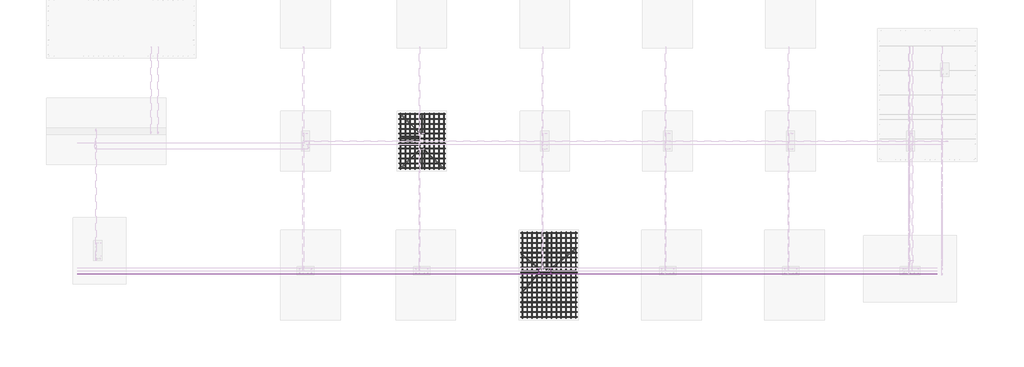
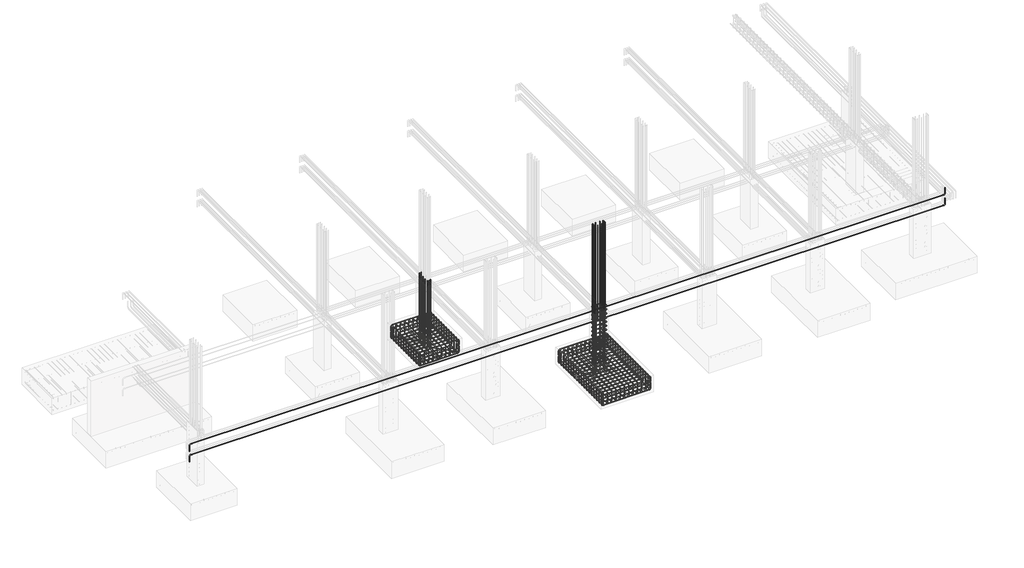
# One storey, part 5 of 18: 30 reinforcing bars.
"""IFC4 building model written with IfcOpenShell, lengths in millimetres."""

from ifc_helpers import new_model, si_unit, point, frame, origin, place, context, project, spatial, polyline, circle_curve, trimmed, segment, composite_curve, source, transform, mapped, element, save
from ifc_brep_helpers import swept_disk

model = new_model("IFC4")

# Units and contexts
model_context = context("Model", 3, world=origin())
ifc_project = project(units=[si_unit("LENGTHUNIT", "METRE", prefix="MILLI")], contexts=[model_context])

# Site, building, storey
site = spatial("IfcSite", under=ifc_project)
building = spatial("IfcBuilding", under=site)
storey = spatial("IfcBuildingStorey", under=building, Elevation=-2000.0)

# Reinforcing bars
placement = place(None, origin())
reinforcing_bar_shape = source(origin(), model_context, "Body", "SolidModel", [
    swept_disk(composite_curve([segment(polyline([(-4478.5399692, -834.8555128, -2300.0), (-4478.5399692, -834.8555128, -2486.6)]), True, "CONTINUOUS"), segment(trimmed(circle_curve(frame((-4533.9899692, -834.8555128, -2486.6), z_axis=(0.0, 1.0, 0.0), x_axis=(55.44999999999982, 0.0, 0.0)), 55.45), [point((-4478.5399692, -834.8555128, -2486.6))], [point((-4533.9899692, -834.8555128, -2542.05))], True, "CARTESIAN"), True, "CONTINUOUS"), segment(polyline([(-4533.9899692, -834.8555128, -2542.05), (-5807.1899692, -834.8555128, -2542.05)]), True, "CONTINUOUS"), segment(trimmed(circle_curve(frame((-5807.1899692, -834.8555128, -2486.6), z_axis=(0.0, 1.0, 0.0), x_axis=(0.0, 0.0, -55.45000000000027)), 55.45), [point((-5807.1899692, -834.8555128, -2542.05))], [point((-5862.6399692, -834.8555128, -2486.6))], True, "CARTESIAN"), True, "CONTINUOUS"), segment(polyline([(-5862.6399692, -834.8555128, -2486.6), (-5862.6399692, -834.8555128, -2300.0)]), True, "CONTINUOUS")], self_intersect=False), 7.95),
])
element("IfcReinforcingBar", 1, at=placement, inside=storey, context=model_context, shape_type="MappedRepresentation", body=[
    mapped(reinforcing_bar_shape, transform((0.0, 0.0, 0.0), x_axis=(1.0, 0.0, 0.0), y_axis=(0.0, 1.0, 0.0), z_axis=(0.0, 0.0, 1.0))),
    mapped(reinforcing_bar_shape, transform((0.0, -148.4250709, 0.0), x_axis=(1.0, 0.0, 0.0), y_axis=(0.0, 1.0, 0.0), z_axis=(0.0, 0.0, 1.0))),
    mapped(reinforcing_bar_shape, transform((0.0, -296.8501418, 0.0), x_axis=(1.0, 0.0, 0.0), y_axis=(0.0, 1.0, 0.0), z_axis=(0.0, 0.0, 1.0))),
    mapped(reinforcing_bar_shape, transform((0.0, -445.2752126, 0.0), x_axis=(1.0, 0.0, 0.0), y_axis=(0.0, 1.0, 0.0), z_axis=(0.0, 0.0, 1.0))),
    mapped(reinforcing_bar_shape, transform((0.0, -593.7002835, 0.0), x_axis=(1.0, 0.0, 0.0), y_axis=(0.0, 1.0, 0.0), z_axis=(0.0, 0.0, 1.0))),
    mapped(reinforcing_bar_shape, transform((0.0, -742.1253544, 0.0), x_axis=(1.0, 0.0, 0.0), y_axis=(0.0, 1.0, 0.0), z_axis=(0.0, 0.0, 1.0))),
    mapped(reinforcing_bar_shape, transform((0.0, -890.5504253, 0.0), x_axis=(1.0, 0.0, 0.0), y_axis=(0.0, 1.0, 0.0), z_axis=(0.0, 0.0, 1.0))),
    mapped(reinforcing_bar_shape, transform((0.0, -1038.9754961, 0.0), x_axis=(1.0, 0.0, 0.0), y_axis=(0.0, 1.0, 0.0), z_axis=(0.0, 0.0, 1.0))),
    mapped(reinforcing_bar_shape, transform((0.0, -1187.400567, 0.0), x_axis=(1.0, 0.0, 0.0), y_axis=(0.0, 1.0, 0.0), z_axis=(0.0, 0.0, 1.0))),
    mapped(reinforcing_bar_shape, transform((0.0, -1335.8256379, 0.0), x_axis=(1.0, 0.0, 0.0), y_axis=(0.0, 1.0, 0.0), z_axis=(0.0, 0.0, 1.0))),
    mapped(reinforcing_bar_shape, transform((0.0, -1484.2507088, 0.0), x_axis=(1.0, 0.0, 0.0), y_axis=(0.0, 1.0, 0.0), z_axis=(0.0, 0.0, 1.0))),
    mapped(reinforcing_bar_shape, transform((0.0, -1632.6757796, 0.0), x_axis=(1.0, 0.0, 0.0), y_axis=(0.0, 1.0, 0.0), z_axis=(0.0, 0.0, 1.0))),
])
reinforcing_bar_2_shape = source(origin(), model_context, "Body", "SolidModel", [
    swept_disk(composite_curve([segment(polyline([(-5864.5899692, -834.8555128, -2250.0), (-5864.5899692, -834.8555128, -2102.0)]), True, "CONTINUOUS"), segment(trimmed(circle_curve(frame((-5818.5899692, -834.8555128, -2102.0), z_axis=(0.0, 1.0, 0.0), x_axis=(-46.0, 0.0, 0.0)), 46.0), [point((-5864.5899692, -834.8555128, -2102.0))], [point((-5818.5899692, -834.8555128, -2056.0))], True, "CARTESIAN"), True, "CONTINUOUS"), segment(polyline([(-5818.5899692, -834.8555128, -2056.0), (-4522.5899692, -834.8555128, -2056.0)]), True, "CONTINUOUS"), segment(trimmed(circle_curve(frame((-4522.5899692, -834.8555128, -2102.0), z_axis=(0.0, 1.0, 0.0), x_axis=(0.0, 0.0, 46.0)), 46.0), [point((-4522.5899692, -834.8555128, -2056.0))], [point((-4476.5899692, -834.8555128, -2102.0))], True, "CARTESIAN"), True, "CONTINUOUS"), segment(polyline([(-4476.5899692, -834.8555128, -2102.0), (-4476.5899692, -834.8555128, -2250.0)]), True, "CONTINUOUS")], self_intersect=False), 6.0),
])
element("IfcReinforcingBar", 2, at=placement, inside=storey, context=model_context, shape_type="MappedRepresentation", body=[
    mapped(reinforcing_bar_2_shape, transform((0.0, 0.0, 0.0), x_axis=(1.0, 0.0, 0.0), y_axis=(0.0, 1.0, 0.0), z_axis=(0.0, 0.0, 1.0))),
    mapped(reinforcing_bar_2_shape, transform((0.0, -148.4250709, 0.0), x_axis=(1.0, 0.0, 0.0), y_axis=(0.0, 1.0, 0.0), z_axis=(0.0, 0.0, 1.0))),
    mapped(reinforcing_bar_2_shape, transform((0.0, -296.8501418, 0.0), x_axis=(1.0, 0.0, 0.0), y_axis=(0.0, 1.0, 0.0), z_axis=(0.0, 0.0, 1.0))),
    mapped(reinforcing_bar_2_shape, transform((0.0, -445.2752126, 0.0), x_axis=(1.0, 0.0, 0.0), y_axis=(0.0, 1.0, 0.0), z_axis=(0.0, 0.0, 1.0))),
    mapped(reinforcing_bar_2_shape, transform((0.0, -593.7002835, 0.0), x_axis=(1.0, 0.0, 0.0), y_axis=(0.0, 1.0, 0.0), z_axis=(0.0, 0.0, 1.0))),
    mapped(reinforcing_bar_2_shape, transform((0.0, -742.1253544, 0.0), x_axis=(1.0, 0.0, 0.0), y_axis=(0.0, 1.0, 0.0), z_axis=(0.0, 0.0, 1.0))),
    mapped(reinforcing_bar_2_shape, transform((0.0, -890.5504253, 0.0), x_axis=(1.0, 0.0, 0.0), y_axis=(0.0, 1.0, 0.0), z_axis=(0.0, 0.0, 1.0))),
    mapped(reinforcing_bar_2_shape, transform((0.0, -1038.9754961, 0.0), x_axis=(1.0, 0.0, 0.0), y_axis=(0.0, 1.0, 0.0), z_axis=(0.0, 0.0, 1.0))),
    mapped(reinforcing_bar_2_shape, transform((0.0, -1187.400567, 0.0), x_axis=(1.0, 0.0, 0.0), y_axis=(0.0, 1.0, 0.0), z_axis=(0.0, 0.0, 1.0))),
    mapped(reinforcing_bar_2_shape, transform((0.0, -1335.8256379, 0.0), x_axis=(1.0, 0.0, 0.0), y_axis=(0.0, 1.0, 0.0), z_axis=(0.0, 0.0, 1.0))),
    mapped(reinforcing_bar_2_shape, transform((0.0, -1484.2507088, 0.0), x_axis=(1.0, 0.0, 0.0), y_axis=(0.0, 1.0, 0.0), z_axis=(0.0, 0.0, 1.0))),
    mapped(reinforcing_bar_2_shape, transform((0.0, -1632.6757796, 0.0), x_axis=(1.0, 0.0, 0.0), y_axis=(0.0, 1.0, 0.0), z_axis=(0.0, 0.0, 1.0))),
])
reinforcing_bar_3_shape = source(origin(), model_context, "Body", "SolidModel", [
    swept_disk(composite_curve([segment(polyline([(-5818.4091864, -811.9600376, -2322.6684255), (-5818.4091864, -811.9600376, -2470.6684255)]), True, "CONTINUOUS"), segment(trimmed(circle_curve(frame((-5818.4091864, -857.9600376, -2470.6684255), z_axis=(-1.0, 0.0, 0.0), x_axis=(0.0, 46.0, 0.0)), 46.0), [point((-5818.4091864, -811.9600376, -2470.6684255))], [point((-5818.4091864, -857.9600376, -2516.6684255))], True, "CARTESIAN"), True, "CONTINUOUS"), segment(polyline([(-5818.4091864, -857.9600376, -2516.6684255), (-5818.4091864, -2453.9600376, -2516.6684255)]), True, "CONTINUOUS"), segment(trimmed(circle_curve(frame((-5818.4091864, -2453.9600376, -2470.6684255), z_axis=(-1.0, 0.0, 0.0), x_axis=(0.0, 0.0, -46.0)), 46.0), [point((-5818.4091864, -2453.9600376, -2516.6684255))], [point((-5818.4091864, -2499.9600376, -2470.6684255))], True, "CARTESIAN"), True, "CONTINUOUS"), segment(polyline([(-5818.4091864, -2499.9600376, -2470.6684255), (-5818.4091864, -2499.9600376, -2322.6684255)]), True, "CONTINUOUS")], self_intersect=False), 6.0),
])
element("IfcReinforcingBar", 3, at=placement, inside=storey, context=model_context, shape_type="MappedRepresentation", body=[
    mapped(reinforcing_bar_3_shape, transform((0.0, 0.0, 0.0), x_axis=(1.0, 0.0, 0.0), y_axis=(0.0, 1.0, 0.0), z_axis=(0.0, 0.0, 1.0))),
    mapped(reinforcing_bar_3_shape, transform((144.8687847, 0.0, 0.0), x_axis=(1.0, 0.0, 0.0), y_axis=(0.0, 1.0, 0.0), z_axis=(0.0, 0.0, 1.0))),
    mapped(reinforcing_bar_3_shape, transform((289.7375694, 0.0, 0.0), x_axis=(1.0, 0.0, 0.0), y_axis=(0.0, 1.0, 0.0), z_axis=(0.0, 0.0, 1.0))),
    mapped(reinforcing_bar_3_shape, transform((434.6063541, 0.0, 0.0), x_axis=(1.0, 0.0, 0.0), y_axis=(0.0, 1.0, 0.0), z_axis=(0.0, 0.0, 1.0))),
    mapped(reinforcing_bar_3_shape, transform((579.4751388, 0.0, 0.0), x_axis=(1.0, 0.0, 0.0), y_axis=(0.0, 1.0, 0.0), z_axis=(0.0, 0.0, 1.0))),
    mapped(reinforcing_bar_3_shape, transform((724.3439235, 0.0, 0.0), x_axis=(1.0, 0.0, 0.0), y_axis=(0.0, 1.0, 0.0), z_axis=(0.0, 0.0, 1.0))),
    mapped(reinforcing_bar_3_shape, transform((869.2127082, 0.0, 0.0), x_axis=(1.0, 0.0, 0.0), y_axis=(0.0, 1.0, 0.0), z_axis=(0.0, 0.0, 1.0))),
    mapped(reinforcing_bar_3_shape, transform((1014.0814929, 0.0, 0.0), x_axis=(1.0, 0.0, 0.0), y_axis=(0.0, 1.0, 0.0), z_axis=(0.0, 0.0, 1.0))),
    mapped(reinforcing_bar_3_shape, transform((1158.9502776, 0.0, 0.0), x_axis=(1.0, 0.0, 0.0), y_axis=(0.0, 1.0, 0.0), z_axis=(0.0, 0.0, 1.0))),
    mapped(reinforcing_bar_3_shape, transform((1303.8190623, 0.0, 0.0), x_axis=(1.0, 0.0, 0.0), y_axis=(0.0, 1.0, 0.0), z_axis=(0.0, 0.0, 1.0))),
])
reinforcing_bar_4_shape = source(origin(), model_context, "Body", "SolidModel", [
    swept_disk(composite_curve([segment(polyline([(-4512.6669522, -811.9600376, -2276.6677805), (-4512.6669522, -811.9600376, -2128.6677805)]), True, "CONTINUOUS"), segment(trimmed(circle_curve(frame((-4512.6669522, -857.9600376, -2128.6677805), z_axis=(1.0, 0.0, 0.0), x_axis=(0.0, 46.0, 0.0)), 46.0), [point((-4512.6669522, -811.9600376, -2128.6677805))], [point((-4512.6669522, -857.9600376, -2082.6677805))], True, "CARTESIAN"), True, "CONTINUOUS"), segment(polyline([(-4512.6669522, -857.9600376, -2082.6677805), (-4512.6669522, -2453.9600376, -2082.6677805)]), True, "CONTINUOUS"), segment(trimmed(circle_curve(frame((-4512.6669522, -2453.9600376, -2128.6677805), z_axis=(1.0, 0.0, 0.0), x_axis=(0.0, 0.0, 46.0)), 46.0), [point((-4512.6669522, -2453.9600376, -2082.6677805))], [point((-4512.6669522, -2499.9600376, -2128.6677805))], True, "CARTESIAN"), True, "CONTINUOUS"), segment(polyline([(-4512.6669522, -2499.9600376, -2128.6677805), (-4512.6669522, -2499.9600376, -2276.6677805)]), True, "CONTINUOUS")], self_intersect=False), 6.0),
])
element("IfcReinforcingBar", 4, at=placement, inside=storey, context=model_context, shape_type="MappedRepresentation", body=[
    mapped(reinforcing_bar_4_shape, transform((0.0, 0.0, 0.0), x_axis=(1.0, 0.0, 0.0), y_axis=(0.0, 1.0, 0.0), z_axis=(0.0, 0.0, 1.0))),
    mapped(reinforcing_bar_4_shape, transform((-145.0824705, 0.0, 0.0), x_axis=(1.0, 0.0, 0.0), y_axis=(0.0, 1.0, 0.0), z_axis=(0.0, 0.0, 1.0))),
    mapped(reinforcing_bar_4_shape, transform((-290.1649409, 0.0, 0.0), x_axis=(1.0, 0.0, 0.0), y_axis=(0.0, 1.0, 0.0), z_axis=(0.0, 0.0, 1.0))),
    mapped(reinforcing_bar_4_shape, transform((-435.2474114, 0.0, 0.0), x_axis=(1.0, 0.0, 0.0), y_axis=(0.0, 1.0, 0.0), z_axis=(0.0, 0.0, 1.0))),
    mapped(reinforcing_bar_4_shape, transform((-580.3298819, 0.0, 0.0), x_axis=(1.0, 0.0, 0.0), y_axis=(0.0, 1.0, 0.0), z_axis=(0.0, 0.0, 1.0))),
    mapped(reinforcing_bar_4_shape, transform((-725.4123523, 0.0, 0.0), x_axis=(1.0, 0.0, 0.0), y_axis=(0.0, 1.0, 0.0), z_axis=(0.0, 0.0, 1.0))),
    mapped(reinforcing_bar_4_shape, transform((-870.4948228, 0.0, 0.0), x_axis=(1.0, 0.0, 0.0), y_axis=(0.0, 1.0, 0.0), z_axis=(0.0, 0.0, 1.0))),
    mapped(reinforcing_bar_4_shape, transform((-1015.5772932, 0.0, 0.0), x_axis=(1.0, 0.0, 0.0), y_axis=(0.0, 1.0, 0.0), z_axis=(0.0, 0.0, 1.0))),
    mapped(reinforcing_bar_4_shape, transform((-1160.6597637, 0.0, 0.0), x_axis=(1.0, 0.0, 0.0), y_axis=(0.0, 1.0, 0.0), z_axis=(0.0, 0.0, 1.0))),
    mapped(reinforcing_bar_4_shape, transform((-1305.7422342, 0.0, 0.0), x_axis=(1.0, 0.0, 0.0), y_axis=(0.0, 1.0, 0.0), z_axis=(0.0, 0.0, 1.0))),
])
reinforcing_bar_5_shape = source(origin(), model_context, "Body", "SolidModel", [
    swept_disk(composite_curve([segment(polyline([(-508.2940057, -4415.5752408, -2300.0), (-508.2940057, -4415.5752408, -2486.6)]), True, "CONTINUOUS"), segment(trimmed(circle_curve(frame((-563.7440057, -4415.5752408, -2486.6), z_axis=(0.0, 1.0, 0.0), x_axis=(55.44999999999999, 0.0, 0.0)), 55.45), [point((-508.2940057, -4415.5752408, -2486.6))], [point((-563.7440057, -4415.5752408, -2542.05))], True, "CARTESIAN"), True, "CONTINUOUS"), segment(polyline([(-563.7440057, -4415.5752408, -2542.05), (-2136.9440057, -4415.5752408, -2542.05)]), True, "CONTINUOUS"), segment(trimmed(circle_curve(frame((-2136.9440057, -4415.5752408, -2486.6), z_axis=(0.0, 1.0, 0.0), x_axis=(0.0, 0.0, -55.45000000000027)), 55.45), [point((-2136.9440057, -4415.5752408, -2542.05))], [point((-2192.3940057, -4415.5752408, -2486.6))], True, "CARTESIAN"), True, "CONTINUOUS"), segment(polyline([(-2192.3940057, -4415.5752408, -2486.6), (-2192.3940057, -4415.5752408, -2300.0)]), True, "CONTINUOUS")], self_intersect=False), 7.95),
])
element("IfcReinforcingBar", 5, at=placement, inside=storey, context=model_context, shape_type="MappedRepresentation", body=[
    mapped(reinforcing_bar_5_shape, transform((0.0, 0.0, 0.0), x_axis=(1.0, 0.0, 0.0), y_axis=(0.0, 1.0, 0.0), z_axis=(0.0, 0.0, 1.0))),
    mapped(reinforcing_bar_5_shape, transform((0.0, -148.9809282, 0.0), x_axis=(1.0, 0.0, 0.0), y_axis=(0.0, 1.0, 0.0), z_axis=(0.0, 0.0, 1.0))),
    mapped(reinforcing_bar_5_shape, transform((0.0, -297.9618564, 0.0), x_axis=(1.0, 0.0, 0.0), y_axis=(0.0, 1.0, 0.0), z_axis=(0.0, 0.0, 1.0))),
    mapped(reinforcing_bar_5_shape, transform((0.0, -446.9427846, 0.0), x_axis=(1.0, 0.0, 0.0), y_axis=(0.0, 1.0, 0.0), z_axis=(0.0, 0.0, 1.0))),
    mapped(reinforcing_bar_5_shape, transform((0.0, -595.9237129, 0.0), x_axis=(1.0, 0.0, 0.0), y_axis=(0.0, 1.0, 0.0), z_axis=(0.0, 0.0, 1.0))),
    mapped(reinforcing_bar_5_shape, transform((0.0, -744.9046411, 0.0), x_axis=(1.0, 0.0, 0.0), y_axis=(0.0, 1.0, 0.0), z_axis=(0.0, 0.0, 1.0))),
    mapped(reinforcing_bar_5_shape, transform((0.0, -893.8855693, 0.0), x_axis=(1.0, 0.0, 0.0), y_axis=(0.0, 1.0, 0.0), z_axis=(0.0, 0.0, 1.0))),
    mapped(reinforcing_bar_5_shape, transform((0.0, -1042.8664975, 0.0), x_axis=(1.0, 0.0, 0.0), y_axis=(0.0, 1.0, 0.0), z_axis=(0.0, 0.0, 1.0))),
    mapped(reinforcing_bar_5_shape, transform((0.0, -1191.8474257, 0.0), x_axis=(1.0, 0.0, 0.0), y_axis=(0.0, 1.0, 0.0), z_axis=(0.0, 0.0, 1.0))),
    mapped(reinforcing_bar_5_shape, transform((0.0, -1340.8283539, 0.0), x_axis=(1.0, 0.0, 0.0), y_axis=(0.0, 1.0, 0.0), z_axis=(0.0, 0.0, 1.0))),
    mapped(reinforcing_bar_5_shape, transform((0.0, -1489.8092821, 0.0), x_axis=(1.0, 0.0, 0.0), y_axis=(0.0, 1.0, 0.0), z_axis=(0.0, 0.0, 1.0))),
    mapped(reinforcing_bar_5_shape, transform((0.0, -1638.7902103, 0.0), x_axis=(1.0, 0.0, 0.0), y_axis=(0.0, 1.0, 0.0), z_axis=(0.0, 0.0, 1.0))),
    mapped(reinforcing_bar_5_shape, transform((0.0, -1787.7711386, 0.0), x_axis=(1.0, 0.0, 0.0), y_axis=(0.0, 1.0, 0.0), z_axis=(0.0, 0.0, 1.0))),
    mapped(reinforcing_bar_5_shape, transform((0.0, -1936.7520668, 0.0), x_axis=(1.0, 0.0, 0.0), y_axis=(0.0, 1.0, 0.0), z_axis=(0.0, 0.0, 1.0))),
    mapped(reinforcing_bar_5_shape, transform((0.0, -2085.732995, 0.0), x_axis=(1.0, 0.0, 0.0), y_axis=(0.0, 1.0, 0.0), z_axis=(0.0, 0.0, 1.0))),
    mapped(reinforcing_bar_5_shape, transform((0.0, -2234.7139232, 0.0), x_axis=(1.0, 0.0, 0.0), y_axis=(0.0, 1.0, 0.0), z_axis=(0.0, 0.0, 1.0))),
    mapped(reinforcing_bar_5_shape, transform((0.0, -2383.6948514, 0.0), x_axis=(1.0, 0.0, 0.0), y_axis=(0.0, 1.0, 0.0), z_axis=(0.0, 0.0, 1.0))),
    mapped(reinforcing_bar_5_shape, transform((0.0, -2532.6757796, 0.0), x_axis=(1.0, 0.0, 0.0), y_axis=(0.0, 1.0, 0.0), z_axis=(0.0, 0.0, 1.0))),
])
reinforcing_bar_6_shape = source(origin(), model_context, "Body", "SolidModel", [
    swept_disk(composite_curve([segment(polyline([(-2194.3440057, -4415.5752408, -2250.0), (-2194.3440057, -4415.5752408, -2102.0)]), True, "CONTINUOUS"), segment(trimmed(circle_curve(frame((-2148.3440057, -4415.5752408, -2102.0), z_axis=(0.0, 1.0, 0.0), x_axis=(-46.0, 0.0, 0.0)), 46.0), [point((-2194.3440057, -4415.5752408, -2102.0))], [point((-2148.3440057, -4415.5752408, -2056.0))], True, "CARTESIAN"), True, "CONTINUOUS"), segment(polyline([(-2148.3440057, -4415.5752408, -2056.0), (-552.3440057, -4415.5752408, -2056.0)]), True, "CONTINUOUS"), segment(trimmed(circle_curve(frame((-552.3440057, -4415.5752408, -2102.0), z_axis=(0.0, 1.0, 0.0), x_axis=(0.0, 0.0, 46.0)), 46.0), [point((-552.3440057, -4415.5752408, -2056.0))], [point((-506.3440057, -4415.5752408, -2102.0))], True, "CARTESIAN"), True, "CONTINUOUS"), segment(polyline([(-506.3440057, -4415.5752408, -2102.0), (-506.3440057, -4415.5752408, -2250.0)]), True, "CONTINUOUS")], self_intersect=False), 6.0),
])
element("IfcReinforcingBar", 6, at=placement, inside=storey, context=model_context, shape_type="MappedRepresentation", body=[
    mapped(reinforcing_bar_6_shape, transform((0.0, 0.0, 0.0), x_axis=(1.0, 0.0, 0.0), y_axis=(0.0, 1.0, 0.0), z_axis=(0.0, 0.0, 1.0))),
    mapped(reinforcing_bar_6_shape, transform((0.0, -148.9809282, 0.0), x_axis=(1.0, 0.0, 0.0), y_axis=(0.0, 1.0, 0.0), z_axis=(0.0, 0.0, 1.0))),
    mapped(reinforcing_bar_6_shape, transform((0.0, -297.9618564, 0.0), x_axis=(1.0, 0.0, 0.0), y_axis=(0.0, 1.0, 0.0), z_axis=(0.0, 0.0, 1.0))),
    mapped(reinforcing_bar_6_shape, transform((0.0, -446.9427846, 0.0), x_axis=(1.0, 0.0, 0.0), y_axis=(0.0, 1.0, 0.0), z_axis=(0.0, 0.0, 1.0))),
    mapped(reinforcing_bar_6_shape, transform((0.0, -595.9237129, 0.0), x_axis=(1.0, 0.0, 0.0), y_axis=(0.0, 1.0, 0.0), z_axis=(0.0, 0.0, 1.0))),
    mapped(reinforcing_bar_6_shape, transform((0.0, -744.9046411, 0.0), x_axis=(1.0, 0.0, 0.0), y_axis=(0.0, 1.0, 0.0), z_axis=(0.0, 0.0, 1.0))),
    mapped(reinforcing_bar_6_shape, transform((0.0, -893.8855693, 0.0), x_axis=(1.0, 0.0, 0.0), y_axis=(0.0, 1.0, 0.0), z_axis=(0.0, 0.0, 1.0))),
    mapped(reinforcing_bar_6_shape, transform((0.0, -1042.8664975, 0.0), x_axis=(1.0, 0.0, 0.0), y_axis=(0.0, 1.0, 0.0), z_axis=(0.0, 0.0, 1.0))),
    mapped(reinforcing_bar_6_shape, transform((0.0, -1191.8474257, 0.0), x_axis=(1.0, 0.0, 0.0), y_axis=(0.0, 1.0, 0.0), z_axis=(0.0, 0.0, 1.0))),
    mapped(reinforcing_bar_6_shape, transform((0.0, -1340.8283539, 0.0), x_axis=(1.0, 0.0, 0.0), y_axis=(0.0, 1.0, 0.0), z_axis=(0.0, 0.0, 1.0))),
    mapped(reinforcing_bar_6_shape, transform((0.0, -1489.8092821, 0.0), x_axis=(1.0, 0.0, 0.0), y_axis=(0.0, 1.0, 0.0), z_axis=(0.0, 0.0, 1.0))),
    mapped(reinforcing_bar_6_shape, transform((0.0, -1638.7902103, 0.0), x_axis=(1.0, 0.0, 0.0), y_axis=(0.0, 1.0, 0.0), z_axis=(0.0, 0.0, 1.0))),
    mapped(reinforcing_bar_6_shape, transform((0.0, -1787.7711386, 0.0), x_axis=(1.0, 0.0, 0.0), y_axis=(0.0, 1.0, 0.0), z_axis=(0.0, 0.0, 1.0))),
    mapped(reinforcing_bar_6_shape, transform((0.0, -1936.7520668, 0.0), x_axis=(1.0, 0.0, 0.0), y_axis=(0.0, 1.0, 0.0), z_axis=(0.0, 0.0, 1.0))),
    mapped(reinforcing_bar_6_shape, transform((0.0, -2085.732995, 0.0), x_axis=(1.0, 0.0, 0.0), y_axis=(0.0, 1.0, 0.0), z_axis=(0.0, 0.0, 1.0))),
    mapped(reinforcing_bar_6_shape, transform((0.0, -2234.7139232, 0.0), x_axis=(1.0, 0.0, 0.0), y_axis=(0.0, 1.0, 0.0), z_axis=(0.0, 0.0, 1.0))),
    mapped(reinforcing_bar_6_shape, transform((0.0, -2383.6948514, 0.0), x_axis=(1.0, 0.0, 0.0), y_axis=(0.0, 1.0, 0.0), z_axis=(0.0, 0.0, 1.0))),
    mapped(reinforcing_bar_6_shape, transform((0.0, -2532.6757796, 0.0), x_axis=(1.0, 0.0, 0.0), y_axis=(0.0, 1.0, 0.0), z_axis=(0.0, 0.0, 1.0))),
])
reinforcing_bar_7_shape = source(origin(), model_context, "Body", "SolidModel", [
    swept_disk(composite_curve([segment(polyline([(-2148.1632229, -4392.6797656, -2322.6684255), (-2148.1632229, -4392.6797656, -2470.6684255)]), True, "CONTINUOUS"), segment(trimmed(circle_curve(frame((-2148.1632229, -4438.6797656, -2470.6684255), z_axis=(-1.0, 0.0, 0.0), x_axis=(0.0, 46.0, 0.0)), 46.0), [point((-2148.1632229, -4392.6797656, -2470.6684255))], [point((-2148.1632229, -4438.6797656, -2516.6684255))], True, "CARTESIAN"), True, "CONTINUOUS"), segment(polyline([(-2148.1632229, -4438.6797656, -2516.6684255), (-2148.1632229, -6934.6797656, -2516.6684255)]), True, "CONTINUOUS"), segment(trimmed(circle_curve(frame((-2148.1632229, -6934.6797656, -2470.6684255), z_axis=(-1.0, 0.0, 0.0), x_axis=(0.0, 0.0, -46.0)), 46.0), [point((-2148.1632229, -6934.6797656, -2516.6684255))], [point((-2148.1632229, -6980.6797656, -2470.6684255))], True, "CARTESIAN"), True, "CONTINUOUS"), segment(polyline([(-2148.1632229, -6980.6797656, -2470.6684255), (-2148.1632229, -6980.6797656, -2322.6684255)]), True, "CONTINUOUS")], self_intersect=False), 6.0),
])
element("IfcReinforcingBar", 7, at=placement, inside=storey, context=model_context, shape_type="MappedRepresentation", body=[
    mapped(reinforcing_bar_7_shape, transform((0.0, 0.0, 0.0), x_axis=(1.0, 0.0, 0.0), y_axis=(0.0, 1.0, 0.0), z_axis=(0.0, 0.0, 1.0))),
    mapped(reinforcing_bar_7_shape, transform((145.8017329, 0.0, 0.0), x_axis=(1.0, 0.0, 0.0), y_axis=(0.0, 1.0, 0.0), z_axis=(0.0, 0.0, 1.0))),
    mapped(reinforcing_bar_7_shape, transform((291.6034659, 0.0, 0.0), x_axis=(1.0, 0.0, 0.0), y_axis=(0.0, 1.0, 0.0), z_axis=(0.0, 0.0, 1.0))),
    mapped(reinforcing_bar_7_shape, transform((437.4051988, 0.0, 0.0), x_axis=(1.0, 0.0, 0.0), y_axis=(0.0, 1.0, 0.0), z_axis=(0.0, 0.0, 1.0))),
    mapped(reinforcing_bar_7_shape, transform((583.2069318, 0.0, 0.0), x_axis=(1.0, 0.0, 0.0), y_axis=(0.0, 1.0, 0.0), z_axis=(0.0, 0.0, 1.0))),
    mapped(reinforcing_bar_7_shape, transform((729.0086647, 0.0, 0.0), x_axis=(1.0, 0.0, 0.0), y_axis=(0.0, 1.0, 0.0), z_axis=(0.0, 0.0, 1.0))),
    mapped(reinforcing_bar_7_shape, transform((874.8103976, 0.0, 0.0), x_axis=(1.0, 0.0, 0.0), y_axis=(0.0, 1.0, 0.0), z_axis=(0.0, 0.0, 1.0))),
    mapped(reinforcing_bar_7_shape, transform((1020.6121306, 0.0, 0.0), x_axis=(1.0, 0.0, 0.0), y_axis=(0.0, 1.0, 0.0), z_axis=(0.0, 0.0, 1.0))),
    mapped(reinforcing_bar_7_shape, transform((1166.4138635, 0.0, 0.0), x_axis=(1.0, 0.0, 0.0), y_axis=(0.0, 1.0, 0.0), z_axis=(0.0, 0.0, 1.0))),
    mapped(reinforcing_bar_7_shape, transform((1312.2155965, 0.0, 0.0), x_axis=(1.0, 0.0, 0.0), y_axis=(0.0, 1.0, 0.0), z_axis=(0.0, 0.0, 1.0))),
    mapped(reinforcing_bar_7_shape, transform((1458.0173294, 0.0, 0.0), x_axis=(1.0, 0.0, 0.0), y_axis=(0.0, 1.0, 0.0), z_axis=(0.0, 0.0, 1.0))),
    mapped(reinforcing_bar_7_shape, transform((1603.8190623, 0.0, 0.0), x_axis=(1.0, 0.0, 0.0), y_axis=(0.0, 1.0, 0.0), z_axis=(0.0, 0.0, 1.0))),
])
reinforcing_bar_8_shape = source(origin(), model_context, "Body", "SolidModel", [
    swept_disk(composite_curve([segment(polyline([(-542.4209887, -4392.6797656, -2276.6677805), (-542.4209887, -4392.6797656, -2128.6677805)]), True, "CONTINUOUS"), segment(trimmed(circle_curve(frame((-542.4209887, -4438.6797656, -2128.6677805), z_axis=(1.0, 0.0, 0.0), x_axis=(0.0, 46.0, 0.0)), 46.0), [point((-542.4209887, -4392.6797656, -2128.6677805))], [point((-542.4209887, -4438.6797656, -2082.6677805))], True, "CARTESIAN"), True, "CONTINUOUS"), segment(polyline([(-542.4209887, -4438.6797656, -2082.6677805), (-542.4209887, -6934.6797656, -2082.6677805)]), True, "CONTINUOUS"), segment(trimmed(circle_curve(frame((-542.4209887, -6934.6797656, -2128.6677805), z_axis=(1.0, 0.0, 0.0), x_axis=(0.0, 0.0, 46.0)), 46.0), [point((-542.4209887, -6934.6797656, -2082.6677805))], [point((-542.4209887, -6980.6797656, -2128.6677805))], True, "CARTESIAN"), True, "CONTINUOUS"), segment(polyline([(-542.4209887, -6980.6797656, -2128.6677805), (-542.4209887, -6980.6797656, -2276.6677805)]), True, "CONTINUOUS")], self_intersect=False), 6.0),
])
element("IfcReinforcingBar", 8, at=placement, inside=storey, context=model_context, shape_type="MappedRepresentation", body=[
    mapped(reinforcing_bar_8_shape, transform((0.0, 0.0, 0.0), x_axis=(1.0, 0.0, 0.0), y_axis=(0.0, 1.0, 0.0), z_axis=(0.0, 0.0, 1.0))),
    mapped(reinforcing_bar_8_shape, transform((-145.9765667, 0.0, 0.0), x_axis=(1.0, 0.0, 0.0), y_axis=(0.0, 1.0, 0.0), z_axis=(0.0, 0.0, 1.0))),
    mapped(reinforcing_bar_8_shape, transform((-291.9531335, 0.0, 0.0), x_axis=(1.0, 0.0, 0.0), y_axis=(0.0, 1.0, 0.0), z_axis=(0.0, 0.0, 1.0))),
    mapped(reinforcing_bar_8_shape, transform((-437.9297002, 0.0, 0.0), x_axis=(1.0, 0.0, 0.0), y_axis=(0.0, 1.0, 0.0), z_axis=(0.0, 0.0, 1.0))),
    mapped(reinforcing_bar_8_shape, transform((-583.906267, 0.0, 0.0), x_axis=(1.0, 0.0, 0.0), y_axis=(0.0, 1.0, 0.0), z_axis=(0.0, 0.0, 1.0))),
    mapped(reinforcing_bar_8_shape, transform((-729.8828337, 0.0, 0.0), x_axis=(1.0, 0.0, 0.0), y_axis=(0.0, 1.0, 0.0), z_axis=(0.0, 0.0, 1.0))),
    mapped(reinforcing_bar_8_shape, transform((-875.8594005, 0.0, 0.0), x_axis=(1.0, 0.0, 0.0), y_axis=(0.0, 1.0, 0.0), z_axis=(0.0, 0.0, 1.0))),
    mapped(reinforcing_bar_8_shape, transform((-1021.8359672, 0.0, 0.0), x_axis=(1.0, 0.0, 0.0), y_axis=(0.0, 1.0, 0.0), z_axis=(0.0, 0.0, 1.0))),
    mapped(reinforcing_bar_8_shape, transform((-1167.8125339, 0.0, 0.0), x_axis=(1.0, 0.0, 0.0), y_axis=(0.0, 1.0, 0.0), z_axis=(0.0, 0.0, 1.0))),
    mapped(reinforcing_bar_8_shape, transform((-1313.7891007, 0.0, 0.0), x_axis=(1.0, 0.0, 0.0), y_axis=(0.0, 1.0, 0.0), z_axis=(0.0, 0.0, 1.0))),
    mapped(reinforcing_bar_8_shape, transform((-1459.7656674, 0.0, 0.0), x_axis=(1.0, 0.0, 0.0), y_axis=(0.0, 1.0, 0.0), z_axis=(0.0, 0.0, 1.0))),
    mapped(reinforcing_bar_8_shape, transform((-1605.7422342, 0.0, 0.0), x_axis=(1.0, 0.0, 0.0), y_axis=(0.0, 1.0, 0.0), z_axis=(0.0, 0.0, 1.0))),
])
reinforcing_bar_9_shape = source(origin(), model_context, "Body", "SolidModel", [
    swept_disk(composite_curve([segment(polyline([(-1360.4315175, -5535.5091206, -34.0), (-1304.0960659, -5479.1736689, -34.0)]), True, "CONTINUOUS"), segment(trimmed(circle_curve(frame((-1283.5899692, -5499.6797656, -34.0), z_axis=(0.0, 0.0, -1.0), x_axis=(-20.506096699999944, 20.506096699999944, 0.0)), 29.0), [point((-1304.0960659, -5479.1736689, -34.0))], [point((-1254.5899692, -5499.6797656, -34.0))], True, "CARTESIAN"), True, "CONTINUOUS"), segment(polyline([(-1254.5899692, -5499.6797656, -34.0), (-1254.5899692, -5623.6797656, -34.0)]), True, "CONTINUOUS"), segment(trimmed(circle_curve(frame((-1283.5899692, -5623.6797656, -34.0), z_axis=(0.0, 0.0, -1.0), x_axis=(29.0, 0.0, 0.0)), 29.0), [point((-1254.5899692, -5623.6797656, -34.0))], [point((-1283.5899692, -5652.6797656, -34.0))], True, "CARTESIAN"), True, "CONTINUOUS"), segment(polyline([(-1283.5899692, -5652.6797656, -34.0), (-1657.5899692, -5652.6797656, -34.0)]), True, "CONTINUOUS"), segment(trimmed(circle_curve(frame((-1657.5899692, -5623.707741, -32.7265044), z_axis=(0.0, 0.043913640913297095, -0.9990353307775146), x_axis=(0.0, -28.972024599999713, -1.2734955999999968)), 29.0), [point((-1657.5899692, -5652.6797656, -34.0))], [point((-1686.5899692, -5623.707741, -32.7265044))], True, "CARTESIAN"), True, "CONTINUOUS"), segment(polyline([(-1686.5899692, -5623.707741, -32.7265044), (-1686.5899692, -5499.6517902, -27.2734956)]), True, "CONTINUOUS"), segment(trimmed(circle_curve(frame((-1657.5899692, -5499.6517902, -27.2734956), z_axis=(0.0, 0.043913640913297095, -0.9990353307775146), x_axis=(-29.0, 0.0, 0.0)), 29.0), [point((-1686.5899692, -5499.6517902, -27.2734956))], [point((-1657.5899692, -5470.6797656, -26.0))], True, "CARTESIAN"), True, "CONTINUOUS"), segment(polyline([(-1657.5899692, -5470.6797656, -26.0), (-1283.5899692, -5470.6797656, -26.0)]), True, "CONTINUOUS"), segment(trimmed(circle_curve(frame((-1283.5899692, -5499.6797656, -26.0), z_axis=(0.0, 0.0, -1.0), x_axis=(0.0, 29.0, 0.0)), 29.0), [point((-1283.5899692, -5470.6797656, -26.0))], [point((-1263.0838726, -5520.1858622, -26.0))], True, "CARTESIAN"), True, "CONTINUOUS"), segment(polyline([(-1263.0838726, -5520.1858622, -26.0), (-1319.4193242, -5576.5213139, -26.0)]), True, "CONTINUOUS")], self_intersect=False), 4.0),
])
element("IfcReinforcingBar", 9, at=placement, inside=storey, context=model_context, shape_type="MappedRepresentation", body=[
    mapped(reinforcing_bar_9_shape, transform((0.0, 0.0, 0.0), x_axis=(1.0, 0.0, 0.0), y_axis=(0.0, 1.0, 0.0), z_axis=(0.0, 0.0, 1.0))),
    mapped(reinforcing_bar_9_shape, transform((0.0, 0.0, -148.6153846), x_axis=(1.0, 0.0, 0.0), y_axis=(0.0, 1.0, 0.0), z_axis=(0.0, 0.0, 1.0))),
    mapped(reinforcing_bar_9_shape, transform((0.0, 0.0, -297.2307692), x_axis=(1.0, 0.0, 0.0), y_axis=(0.0, 1.0, 0.0), z_axis=(0.0, 0.0, 1.0))),
    mapped(reinforcing_bar_9_shape, transform((0.0, 0.0, -445.8461538), x_axis=(1.0, 0.0, 0.0), y_axis=(0.0, 1.0, 0.0), z_axis=(0.0, 0.0, 1.0))),
    mapped(reinforcing_bar_9_shape, transform((0.0, 0.0, -594.4615385), x_axis=(1.0, 0.0, 0.0), y_axis=(0.0, 1.0, 0.0), z_axis=(0.0, 0.0, 1.0))),
    mapped(reinforcing_bar_9_shape, transform((0.0, 0.0, -743.0769231), x_axis=(1.0, 0.0, 0.0), y_axis=(0.0, 1.0, 0.0), z_axis=(0.0, 0.0, 1.0))),
    mapped(reinforcing_bar_9_shape, transform((0.0, 0.0, -891.6923077), x_axis=(1.0, 0.0, 0.0), y_axis=(0.0, 1.0, 0.0), z_axis=(0.0, 0.0, 1.0))),
    mapped(reinforcing_bar_9_shape, transform((0.0, 0.0, -1040.3076923), x_axis=(1.0, 0.0, 0.0), y_axis=(0.0, 1.0, 0.0), z_axis=(0.0, 0.0, 1.0))),
    mapped(reinforcing_bar_9_shape, transform((0.0, 0.0, -1188.9230769), x_axis=(1.0, 0.0, 0.0), y_axis=(0.0, 1.0, 0.0), z_axis=(0.0, 0.0, 1.0))),
    mapped(reinforcing_bar_9_shape, transform((0.0, 0.0, -1337.5384615), x_axis=(1.0, 0.0, 0.0), y_axis=(0.0, 1.0, 0.0), z_axis=(0.0, 0.0, 1.0))),
    mapped(reinforcing_bar_9_shape, transform((0.0, 0.0, -1486.1538462), x_axis=(1.0, 0.0, 0.0), y_axis=(0.0, 1.0, 0.0), z_axis=(0.0, 0.0, 1.0))),
    mapped(reinforcing_bar_9_shape, transform((0.0, 0.0, -1634.7692308), x_axis=(1.0, 0.0, 0.0), y_axis=(0.0, 1.0, 0.0), z_axis=(0.0, 0.0, 1.0))),
    mapped(reinforcing_bar_9_shape, transform((0.0, 0.0, -1783.3846154), x_axis=(1.0, 0.0, 0.0), y_axis=(0.0, 1.0, 0.0), z_axis=(0.0, 0.0, 1.0))),
    mapped(reinforcing_bar_9_shape, transform((0.0, 0.0, -1932.0), x_axis=(1.0, 0.0, 0.0), y_axis=(0.0, 1.0, 0.0), z_axis=(0.0, 0.0, 1.0))),
])
element("IfcReinforcingBar", 10, at=placement, inside=storey, context=model_context, shape_type="SolidModel", body=[
    swept_disk(composite_curve([segment(polyline([(-2173.6233429, -5063.6864072, -2480.0), (-1700.4558049, -5460.7211138, -2480.0)]), True, "CONTINUOUS"), segment(trimmed(circle_curve(frame((-1700.4558049, -5460.7211138, -2412.5), z_axis=(-0.6427876096865429, -0.766044443118975, 0.0), x_axis=(0.0, 0.0, -67.5)), 67.5), [point((-1700.4558049, -5460.7211138, -2480.0))], [point((-1648.747805, -5504.1092774, -2412.5))], True, "CARTESIAN"), True, "CONTINUOUS"), segment(polyline([(-1648.747805, -5504.1092774, -2412.5), (-1648.747805, -5504.1092774, -20.0)]), True, "CONTINUOUS")], self_intersect=False), 10.0),
])
element("IfcReinforcingBar", 11, at=placement, inside=storey, context=model_context, shape_type="SolidModel", body=[
    swept_disk(composite_curve([segment(polyline([(-2177.6576621, -5559.3632831, -2480.0), (-1705.107931, -5559.3632831, -2480.0)]), True, "CONTINUOUS"), segment(trimmed(circle_curve(frame((-1705.107931, -5559.3632831, -2434.0), z_axis=(0.0, -1.0, 0.0), x_axis=(0.0, 0.0, -46.0)), 46.0), [point((-1705.107931, -5559.3632831, -2480.0))], [point((-1659.107931, -5559.3632831, -2434.0))], True, "CARTESIAN"), True, "CONTINUOUS"), segment(polyline([(-1659.107931, -5559.3632831, -2434.0), (-1659.107931, -5559.3632831, -30.0)]), True, "CONTINUOUS")], self_intersect=False), 6.0),
])
element("IfcReinforcingBar", 12, at=placement, inside=storey, context=model_context, shape_type="SolidModel", body=[
    swept_disk(composite_curve([segment(polyline([(-527.0646685, -4861.8897199, -2480.0), (-1240.7241336, -5460.7211138, -2480.0)]), True, "CONTINUOUS"), segment(trimmed(circle_curve(frame((-1240.7241336, -5460.7211138, -2412.5), z_axis=(-0.6427876096865429, 0.766044443118975, 0.0), x_axis=(0.0, 0.0, -67.5)), 67.5), [point((-1240.7241336, -5460.7211138, -2480.0))], [point((-1292.4321335, -5504.1092774, -2412.5))], True, "CARTESIAN"), True, "CONTINUOUS"), segment(polyline([(-1292.4321335, -5504.1092774, -2412.5), (-1292.4321335, -5504.1092774, -20.0)]), True, "CONTINUOUS")], self_intersect=False), 10.0),
])
element("IfcReinforcingBar", 13, at=placement, inside=storey, context=model_context, shape_type="SolidModel", body=[
    swept_disk(composite_curve([segment(polyline([(-2180.6241894, -6231.1040429, -2480.0), (-1693.0317894, -5670.1931504, -2480.0)]), True, "CONTINUOUS"), segment(trimmed(circle_curve(frame((-1693.0317894, -5670.1931504, -2412.5), z_axis=(0.7547095802227678, -0.6560590289905122, 0.0), x_axis=(0.0, 0.0, -67.5)), 67.5), [point((-1693.0317894, -5670.1931504, -2480.0))], [point((-1648.747805, -5619.2502537, -2412.5))], True, "CARTESIAN"), True, "CONTINUOUS"), segment(polyline([(-1648.747805, -5619.2502537, -2412.5), (-1648.747805, -5619.2502537, -20.0)]), True, "CONTINUOUS")], self_intersect=False), 10.0),
])
element("IfcReinforcingBar", 14, at=placement, inside=storey, context=model_context, shape_type="SolidModel", body=[
    swept_disk(composite_curve([segment(polyline([(-523.0303493, -5559.3632831, -2480.0), (-1236.0720074, -5559.3632831, -2480.0)]), True, "CONTINUOUS"), segment(trimmed(circle_curve(frame((-1236.0720074, -5559.3632831, -2434.0), z_axis=(0.0, 1.0, 0.0), x_axis=(0.0, 0.0, -46.0)), 46.0), [point((-1236.0720074, -5559.3632831, -2480.0))], [point((-1282.0720074, -5559.3632831, -2434.0))], True, "CARTESIAN"), True, "CONTINUOUS"), segment(polyline([(-1282.0720074, -5559.3632831, -2434.0), (-1282.0720074, -5559.3632831, -30.0)]), True, "CONTINUOUS")], self_intersect=False), 6.0),
])
reinforcing_bar_10_shape = source(origin(), model_context, "Body", "SolidModel", [
    swept_disk(composite_curve([segment(polyline([(-1543.6420643, -4416.634351, -2480.0), (-1543.6420643, -5449.6419331, -2480.0)]), True, "CONTINUOUS"), segment(trimmed(circle_curve(frame((-1543.6420643, -5449.6419331, -2434.0), z_axis=(-1.0, 0.0, 0.0), x_axis=(0.0, 0.0, -46.0)), 46.0), [point((-1543.6420643, -5449.6419331, -2480.0))], [point((-1543.6420643, -5495.6419331, -2434.0))], True, "CARTESIAN"), True, "CONTINUOUS"), segment(polyline([(-1543.6420643, -5495.6419331, -2434.0), (-1543.6420643, -5495.6419331, -30.0)]), True, "CONTINUOUS")], self_intersect=False), 6.0),
])
element("IfcReinforcingBar", 15, at=placement, inside=storey, context=model_context, shape_type="MappedRepresentation", body=[
    mapped(reinforcing_bar_10_shape, transform((0.0, 0.0, 0.0), x_axis=(1.0, 0.0, 0.0), y_axis=(0.0, 1.0, 0.0), z_axis=(0.0, 0.0, 1.0))),
    mapped(reinforcing_bar_10_shape, transform((144.9594019, 0.0, 0.0), x_axis=(1.0, 0.0, 0.0), y_axis=(0.0, 1.0, 0.0), z_axis=(0.0, 0.0, 1.0))),
])
element("IfcReinforcingBar", 16, at=placement, inside=storey, context=model_context, shape_type="SolidModel", body=[
    swept_disk(composite_curve([segment(polyline([(-5228.3359054, -1423.0839981, -30.0), (-5228.3359054, -1423.0839981, -2431.15)]), True, "CONTINUOUS"), segment(trimmed(circle_curve(frame((-5267.5449764, -1383.874927, -2431.15), z_axis=(0.7071067811865499, 0.7071067811865451, 0.0), x_axis=(39.20907100000022, -39.209071099999846, 0.0)), 55.45), [point((-5228.3359054, -1423.0839981, -2431.15))], [point((-5267.5449764, -1383.874927, -2486.6))], True, "CARTESIAN"), True, "CONTINUOUS"), segment(polyline([(-5267.5449764, -1383.874927, -2486.6), (-5813.39029, -838.0296134, -2486.6)]), True, "CONTINUOUS")], self_intersect=False), 7.95),
])
element("IfcReinforcingBar", 17, at=placement, inside=storey, context=model_context, shape_type="SolidModel", body=[
    swept_disk(composite_curve([segment(polyline([(-5171.037887, -1418.4824597, -30.0), (-5171.037887, -1418.4824597, -2440.6)]), True, "CONTINUOUS"), segment(trimmed(circle_curve(frame((-5171.037887, -1372.4824597, -2440.6), z_axis=(1.0, 0.0, 0.0), x_axis=(0.0, -46.0, 0.0)), 46.0), [point((-5171.037887, -1418.4824597, -2440.6))], [point((-5171.037887, -1372.4824597, -2486.6))], True, "CARTESIAN"), True, "CONTINUOUS"), segment(polyline([(-5171.037887, -1372.4824597, -2486.6), (-5171.037887, -834.8555128, -2486.6)]), True, "CONTINUOUS")], self_intersect=False), 6.0),
])
reinforcing_bar_11_shape = source(origin(), model_context, "Body", "SolidModel", [
    swept_disk(composite_curve([segment(polyline([(-5234.496625, -1776.5422299, -30.0), (-5234.496625, -1776.5422299, -2436.6982733)]), True, "CONTINUOUS"), segment(trimmed(circle_curve(frame((-5280.496625, -1776.5422299, -2436.6982733), z_axis=(0.0, 1.0, 0.0), x_axis=(46.0, 0.0, 0.0)), 46.0), [point((-5234.496625, -1776.5422299, -2436.6982733))], [point((-5280.496625, -1776.5422299, -2482.6982733))], True, "CARTESIAN"), True, "CONTINUOUS"), segment(polyline([(-5280.496625, -1776.5422299, -2482.6982733), (-5817.7267976, -1776.5422299, -2482.6982733)]), True, "CONTINUOUS")], self_intersect=False), 6.0),
])
element("IfcReinforcingBar", 18, at=placement, inside=storey, context=model_context, shape_type="MappedRepresentation", body=[
    mapped(reinforcing_bar_11_shape, transform((0.0, 0.0, 0.0), x_axis=(1.0, 0.0, 0.0), y_axis=(0.0, 1.0, 0.0), z_axis=(0.0, 0.0, 1.0))),
    mapped(reinforcing_bar_11_shape, transform((0.0, 134.2724138, 0.0), x_axis=(1.0, 0.0, 0.0), y_axis=(0.0, 1.0, 0.0), z_axis=(0.0, 0.0, 1.0))),
    mapped(reinforcing_bar_11_shape, transform((0.0, 268.5448277, 0.0), x_axis=(1.0, 0.0, 0.0), y_axis=(0.0, 1.0, 0.0), z_axis=(0.0, 0.0, 1.0))),
])
element("IfcReinforcingBar", 19, at=placement, inside=storey, context=model_context, shape_type="SolidModel", body=[
    swept_disk(composite_curve([segment(polyline([(-5171.037887, -1896.3217695, -30.0), (-5171.037887, -1896.3217695, -2440.6)]), True, "CONTINUOUS"), segment(trimmed(circle_curve(frame((-5171.037887, -1942.3217695, -2440.6), z_axis=(-1.0, 0.0, 0.0), x_axis=(0.0, 46.0, 0.0)), 46.0), [point((-5171.037887, -1896.3217695, -2440.6))], [point((-5171.037887, -1942.3217695, -2486.6))], True, "CARTESIAN"), True, "CONTINUOUS"), segment(polyline([(-5171.037887, -1942.3217695, -2486.6), (-5171.037887, -2479.9487164, -2486.6)]), True, "CONTINUOUS")], self_intersect=False), 6.0),
])
element("IfcReinforcingBar", 20, at=placement, inside=storey, context=model_context, shape_type="SolidModel", body=[
    swept_disk(composite_curve([segment(polyline([(-5228.3359054, -1891.7202311, -30.0), (-5228.3359054, -1891.7202311, -2431.15)]), True, "CONTINUOUS"), segment(trimmed(circle_curve(frame((-5267.5449764, -1930.9293021, -2431.15), z_axis=(-0.7071067811865455, 0.7071067811865496, 0.0), x_axis=(39.20907100000022, 39.209070999999994, 0.0)), 55.45), [point((-5228.3359054, -1891.7202311, -2431.15))], [point((-5267.5449764, -1930.9293021, -2486.6))], True, "CARTESIAN"), True, "CONTINUOUS"), segment(polyline([(-5267.5449764, -1930.9293021, -2486.6), (-5813.39029, -2476.7746158, -2486.6)]), True, "CONTINUOUS")], self_intersect=False), 7.95),
])
element("IfcReinforcingBar", 21, at=placement, inside=storey, context=model_context, shape_type="SolidModel", body=[
    swept_disk(composite_curve([segment(polyline([(-5112.8440331, -1891.7202311, -30.0), (-5112.8440331, -1891.7202311, -2431.15)]), True, "CONTINUOUS"), segment(trimmed(circle_curve(frame((-5073.634962, -1930.9293021, -2431.15), z_axis=(-0.7071067811865546, -0.7071067811865406, 0.0), x_axis=(-39.209071100000074, 39.209070999999994, 0.0)), 55.45), [point((-5112.8440331, -1891.7202311, -2431.15))], [point((-5073.634962, -1930.9293021, -2486.6))], True, "CARTESIAN"), True, "CONTINUOUS"), segment(polyline([(-5073.634962, -1930.9293021, -2486.6), (-4527.7896484, -2476.7746158, -2486.6)]), True, "CONTINUOUS")], self_intersect=False), 7.95),
])
reinforcing_bar_12_shape = source(origin(), model_context, "Body", "SolidModel", [
    swept_disk(composite_curve([segment(polyline([(-15532.6790491, -5651.6797656, -300.2534207), (-15532.6790491, -5651.6797656, -113.6534207)]), True, "CONTINUOUS"), segment(trimmed(circle_curve(frame((-15477.2290491, -5651.6797656, -113.6534207), z_axis=(0.0, 1.0, 0.0), x_axis=(-55.44999999999891, 0.0, 0.0)), 55.45), [point((-15532.6790491, -5651.6797656, -113.6534207))], [point((-15477.2290491, -5651.6797656, -58.2034207))], True, "CARTESIAN"), True, "CONTINUOUS"), segment(polyline([(-15477.2290491, -5651.6797656, -58.2034207), (10261.1848807, -5651.6797656, -58.2034207)]), True, "CONTINUOUS"), segment(trimmed(circle_curve(frame((10261.1848807, -5651.6797656, -2.7534207), z_axis=(0.0, -1.0, 0.0), x_axis=(0.0, 0.0, -55.45)), 55.45), [point((10261.1848807, -5651.6797656, -58.2034207))], [point((10316.6348807, -5651.6797656, -2.7534207))], True, "CARTESIAN"), True, "CONTINUOUS"), segment(polyline([(10316.6348807, -5651.6797656, -2.7534207), (10316.6348807, -5651.6797656, 183.8465793)]), True, "CONTINUOUS")], self_intersect=False), 7.95),
])
element("IfcReinforcingBar", 22, at=placement, inside=storey, context=model_context, shape_type="MappedRepresentation", body=[
    mapped(reinforcing_bar_12_shape, transform((0.0, 0.0, 0.0), x_axis=(1.0, 0.0, 0.0), y_axis=(0.0, 1.0, 0.0), z_axis=(0.0, 0.0, 1.0))),
    mapped(reinforcing_bar_12_shape, transform((0.0, 0.0, -384.9941108), x_axis=(1.0, 0.0, 0.0), y_axis=(0.0, 1.0, 0.0), z_axis=(0.0, 0.0, 1.0))),
])
element("IfcReinforcingBar", 23, at=placement, inside=storey, context=model_context, shape_type="SolidModel", body=[
    swept_disk(composite_curve([segment(polyline([(-1659.1470109, -5560.0856321, -480.0), (-1659.1470109, -5560.0856321, 2970.0)]), True, "CONTINUOUS")], self_intersect=False), 6.0),
])
element("IfcReinforcingBar", 24, at=placement, inside=storey, context=model_context, shape_type="SolidModel", body=[
    swept_disk(composite_curve([segment(polyline([(-1302.4712133, -5504.8316264, -480.0), (-1302.4712133, -5504.8316264, 2970.0)]), True, "CONTINUOUS")], self_intersect=False), 10.0),
])
element("IfcReinforcingBar", 25, at=placement, inside=storey, context=model_context, shape_type="SolidModel", body=[
    swept_disk(composite_curve([segment(polyline([(-1658.7868848, -5619.9726027, -480.0), (-1658.7868848, -5619.9726027, 2970.0)]), True, "CONTINUOUS")], self_intersect=False), 10.0),
])
element("IfcReinforcingBar", 26, at=placement, inside=storey, context=model_context, shape_type="SolidModel", body=[
    swept_disk(composite_curve([segment(polyline([(-1302.4712133, -5619.9726027, -480.0), (-1302.4712133, -5619.9726027, 2970.0)]), True, "CONTINUOUS")], self_intersect=False), 10.0),
])
reinforcing_bar_13_shape = source(origin(), model_context, "Body", "SolidModel", [
    swept_disk(composite_curve([segment(polyline([(-1553.6811441, -5627.6797656, -480.0), (-1553.6811441, -5627.6797656, 2970.0)]), True, "CONTINUOUS")], self_intersect=False), 6.0),
])
element("IfcReinforcingBar", 27, at=placement, inside=storey, context=model_context, shape_type="MappedRepresentation", body=[
    mapped(reinforcing_bar_13_shape, transform((0.0, 0.0, 0.0), x_axis=(1.0, 0.0, 0.0), y_axis=(0.0, 1.0, 0.0), z_axis=(0.0, 0.0, 1.0))),
    mapped(reinforcing_bar_13_shape, transform((144.9594019, 0.0, 0.0), x_axis=(1.0, 0.0, 0.0), y_axis=(0.0, 1.0, 0.0), z_axis=(0.0, 0.0, 1.0))),
])
reinforcing_bar_14_shape = source(origin(), model_context, "Body", "SolidModel", [
    swept_disk(composite_curve([segment(polyline([(-1553.6811441, -5496.3642821, -480.0), (-1553.6811441, -5496.3642821, 2970.0)]), True, "CONTINUOUS")], self_intersect=False), 6.0),
])
element("IfcReinforcingBar", 28, at=placement, inside=storey, context=model_context, shape_type="MappedRepresentation", body=[
    mapped(reinforcing_bar_14_shape, transform((0.0, 0.0, 0.0), x_axis=(1.0, 0.0, 0.0), y_axis=(0.0, 1.0, 0.0), z_axis=(0.0, 0.0, 1.0))),
    mapped(reinforcing_bar_14_shape, transform((144.9594019, 0.0, 0.0), x_axis=(1.0, 0.0, 0.0), y_axis=(0.0, 1.0, 0.0), z_axis=(0.0, 0.0, 1.0))),
])
element("IfcReinforcingBar", 29, at=placement, inside=storey, context=model_context, shape_type="SolidModel", body=[
    swept_disk(composite_curve([segment(polyline([(-1658.7868848, -5504.8316264, -480.0), (-1658.7868848, -5504.8316264, 2970.0)]), True, "CONTINUOUS")], self_intersect=False), 10.0),
])
element("IfcReinforcingBar", 30, at=placement, inside=storey, context=model_context, shape_type="SolidModel", body=[
    swept_disk(composite_curve([segment(polyline([(-1297.1110872, -5560.0856321, -480.0), (-1297.1110872, -5560.0856321, 2970.0)]), True, "CONTINUOUS")], self_intersect=False), 6.0),
])

save(model, "model.ifc")

# Revit data of these elements
# Elements 1, 2, 3, 4, 5, 6, 7, 8, 9, 10, 11, 12, 13, 14, 15, 16, 17, 18, 19, 20, 21, 22, 23, 24, 25, 26, 27, 28, 29, 30 (IfcReinforcingBar)
#   Phase Created = New Construction
